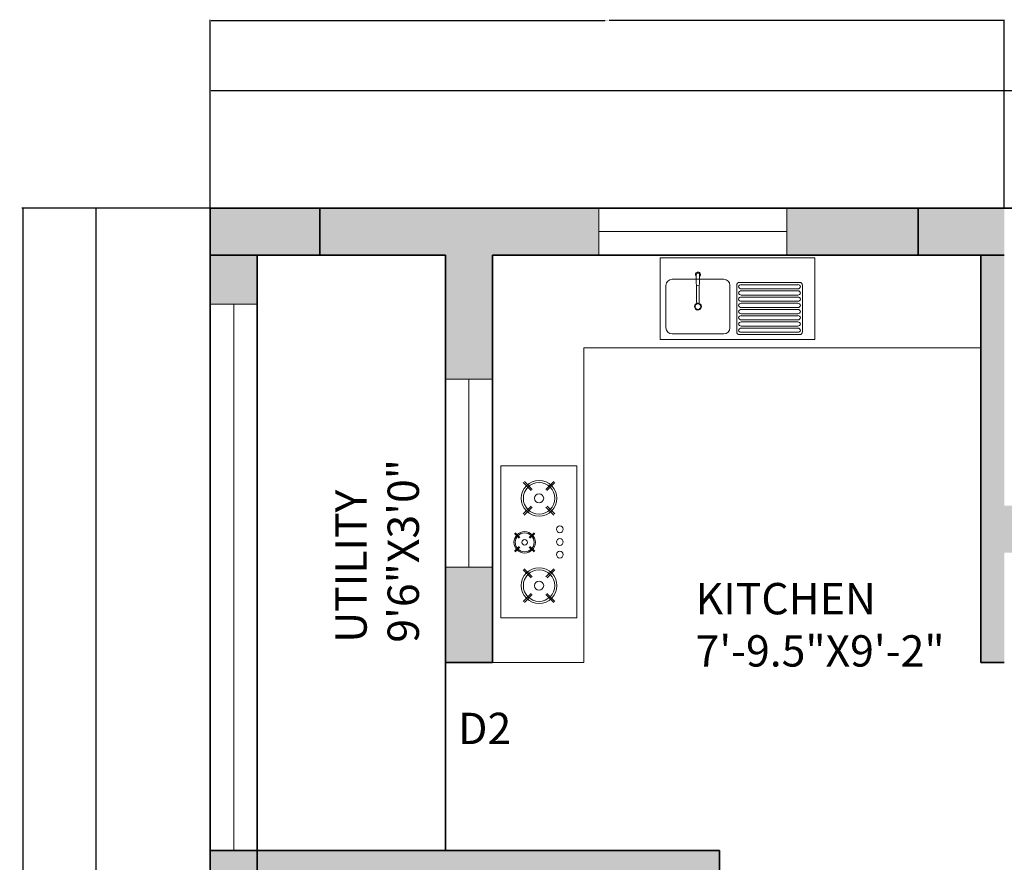
# Model space of a CAD drawing. Units: inches. Extents: x -9 to 505, y -680 to 48.
# Tile 16 of 17: x -9 to 179, y -114 to 48. Entities that reach past the tile are written whole.
import ezdxf

# ---------------------------------------------------------------- set-up
doc = ezdxf.new("R2010")
doc.units = ezdxf.units.IN
doc.header["$MEASUREMENT"] = 0
for name, color, linetype, lineweight in [('A-ANNO-DIMS', 2, 'Continuous', 18), ('A-ANNO-TEXT', 7, 'Continuous', 18), ('A-AREA-IDEN', 7, 'Continuous', 18), ('A-EQPM', 8, 'Continuous', 18), ('A-FLOR-CASE', 8, 'Continuous', 18), ('A-FLOR-FIXT', 9, 'Continuous', 18), ('A-FLOR-HRAL', 4, 'Continuous', 18), ('A-GLAZ', 4, 'Continuous', 18), ('A-WALL', 7, 'Continuous', 35), ('A-WALL-PATT', 251, 'Continuous', 13), ('S-CONC', 7, 'Continuous', 35), ('S-CONC-PATT', 18, 'Continuous', 13)]:
    doc.layers.add(name, color=color, linetype=linetype, lineweight=lineweight)
doc.styles.get("Standard").update_dxf_attribs({"font": 'arial.ttf'})
doc.dimstyles.get("Standard").update_dxf_attribs({"dimtxt": 0.18, "dimasz": 0.18, "dimexe": 0.18, "dimexo": 0.0625, "dimgap": 0.09, "dimtad": 0, "dimtih": 1, "dimtoh": 1, "dimdec": 0, "dimzin": 0, "dimdsep": 46, "dimlunit": 3, "dimtxsty": 'Standard', "dimcen": 0.09, "dimadec": 0, "dimazin": 0, "dimtfac": 1, "dimtdec": 0, "dimtofl": 0, "dimtmove": 0, "dimatfit": 3, "dimfxl": 1, "dimtolj": 1, "dimtzin": 0, "dimarcsym": 0})

# ---------------------------------------------------------------- blocks, each defined once
blk = doc.blocks.new('*D2')
at = {"layer": 'A-ANNO-DIMS', "color": 0, "lineweight": -2, "transparency": 16777216}
for p, q in [((27.26, 11.56), (27.26, 34.2)), ((27.44, 34.02), (235.29, 34.02)), ((468.58, 34.02), (260.74, 34.02)), ((468.76, 11.56), (468.76, 34.2))]:
    blk.add_line(p, q, dxfattribs=at)
at = {"layer": 'A-ANNO-DIMS', "color": 0, "transparency": 16777216}
for points in [[(27.44, 34.05), (27.44, 33.99), (27.26, 34.02)], [(468.58, 34.05), (468.58, 33.99), (468.76, 34.02)]]:
    blk.add_solid(points, dxfattribs=at)
at = {"layer": 'Defpoints', "color": 0, "transparency": 16777216}
for p in [(468.76, 34.02), (27.26, 11.5), (468.76, 11.5)]:
    blk.add_point(p, dxfattribs=at)
at = {"layer": 'A-ANNO-DIMS', "color": 0, "transparency": 16777216, "insert": (248.01, 34.02), "char_height": 6, "attachment_point": 5}
blk.add_mtext('\\A1;36\'-10"', dxfattribs=at)
blk = doc.blocks.new('*D3')
at = {"layer": 'A-ANNO-DIMS', "color": 0, "lineweight": -2, "transparency": 16777216}
for p, q in [((27.2, 11.5), (5.16, 11.5)), ((5.34, 11.32), (5.34, -330.86)), ((5.34, -679.32), (5.34, -337.14)), ((27.2, -679.5), (5.16, -679.5))]:
    blk.add_line(p, q, dxfattribs=at)
at = {"layer": 'A-ANNO-DIMS', "color": 0, "transparency": 16777216}
for points in [[(5.31, 11.32), (5.37, 11.32), (5.34, 11.5)], [(5.31, -679.32), (5.37, -679.32), (5.34, -679.5)]]:
    blk.add_solid(points, dxfattribs=at)
at = {"layer": 'Defpoints', "color": 0, "transparency": 16777216}
for p in [(27.26, 11.5), (5.34, -679.5), (27.26, -679.5)]:
    blk.add_point(p, dxfattribs=at)
at = {"layer": 'A-ANNO-DIMS', "color": 0, "transparency": 16777216, "insert": (5.34, -334), "char_height": 6, "attachment_point": 5}
blk.add_mtext('\\A1;57\'-7"', dxfattribs=at)
blk = doc.blocks.new('WIN-36')
for p, q in [((0, 36), (0, 0)), ((9, 36), (0, 36)), ((4.5, 36), (4.5, 2.23)), ((9, 0), (9, 36)), ((4.5, 2.23), (4.5, 0)), ((0, 0), (9, 0))]:
    blk.add_line(p, q)
blk = doc.blocks.new('SINK-SINGLE-DRAINBOARD')
for p, q in [((0, 0), (0, 15.65)), ((0, 15.65), (29.6, 15.65)), ((29.6, 0), (29.6, 15.65)), ((7.43, 11.55), (2.3, 11.55)), ((12.19, 11.55), (7.57, 11.55)), ((1.13, 10.39), (1.13, 2.25)), ((13.36, 2.25), (13.36, 10.39)), ((14.68, 10.42), (14.68, 1.51)), ((26.71, 10.96), (15.22, 10.96)), ((20.97, 10.52), (15.55, 10.52)), ((20.97, 9.72), (15.55, 9.72)), ((20.97, 10.52), (26.39, 10.52)), ((20.97, 9.72), (26.39, 9.72)), ((27.25, 10.42), (27.25, 1.51)), ((20.97, 9.34), (15.55, 9.34)), ((20.97, 8.53), (15.55, 8.53)), ((20.97, 8.15), (15.55, 8.15)), ((20.97, 9.34), (26.39, 9.34)), ((20.97, 8.53), (26.39, 8.53)), ((20.97, 8.15), (26.39, 8.15)), ((20.97, 7.34), (15.55, 7.34)), ((20.97, 6.96), (15.55, 6.96)), ((20.97, 6.15), (15.55, 6.15)), ((20.97, 5.77), (15.55, 5.77)), ((20.97, 7.34), (26.39, 7.34)), ((20.97, 6.96), (26.39, 6.96)), ((20.97, 6.15), (26.39, 6.15)), ((20.97, 5.77), (26.39, 5.77)), ((20.97, 4.96), (15.55, 4.96)), ((20.97, 4.58), (15.55, 4.58)), ((20.97, 3.78), (15.55, 3.78)), ((20.97, 4.96), (26.39, 4.96)), ((20.97, 4.58), (26.39, 4.58)), ((20.97, 3.78), (26.39, 3.78)), ((20.97, 3.4), (15.55, 3.4)), ((20.97, 2.59), (15.55, 2.59)), ((20.97, 2.21), (15.55, 2.21)), ((20.97, 3.4), (26.39, 3.4)), ((20.97, 2.59), (26.39, 2.59)), ((20.97, 2.21), (26.39, 2.21)), ((2.3, 1.09), (12.19, 1.09)), ((15.22, 0.97), (26.71, 0.97)), ((20.97, 1.4), (15.55, 1.4)), ((20.97, 1.4), (26.39, 1.4)), ((0, 0), (29.6, 0))]:
    blk.add_line(p, q)
for points in [[(6.92, 12.46), (6.92, 10.68)], [(7.57, 12.46), (7.57, 10.68)], [(7, 10.48), (7, 7.2)], [(7.49, 10.48), (7.49, 7.2)]]:
    blk.add_lwpolyline(points)
for radius in [0.674, 0.54]:
    blk.add_circle((7.25, 6.32), radius)
for centre, radius, start, end in [((2.3, 10.39), 1.17, 90, 180), ((7.25, 12.46), 0.485, 311.9018, 228.0982), ((7.25, 12.46), 0.324, 0, 180), ((12.19, 10.39), 1.17, 0, 90), ((7.25, 10.69), 0.324, 182.2198, 357.7802), ((15.22, 10.42), 0.54, 90, 180), ((15.55, 9.99), 0.54, 90, 165.5097), ((15.55, 10.26), 0.54, 194.4903, 270), ((26.39, 9.99), 0.54, 14.4903, 90), ((26.39, 10.26), 0.54, 270, 345.5097), ((26.71, 10.42), 0.54, 0, 90), ((15.55, 8.8), 0.54, 90, 165.5097), ((15.55, 9.07), 0.54, 194.4903, 270), ((15.55, 7.61), 0.54, 90, 165.5097), ((15.55, 7.88), 0.54, 194.4903, 270), ((26.39, 8.8), 0.54, 14.4903, 90), ((26.39, 9.07), 0.54, 270, 345.5097), ((26.39, 7.61), 0.54, 14.4903, 90), ((26.39, 7.88), 0.54, 270, 345.5097), ((7.25, 7.18), 0.244, 174.9463, 5.0537), ((15.55, 6.42), 0.54, 90, 165.5097), ((15.55, 6.69), 0.54, 194.4903, 270), ((15.55, 5.23), 0.54, 90, 165.5097), ((26.39, 6.42), 0.54, 14.4903, 90), ((26.39, 6.69), 0.54, 270, 345.5097), ((26.39, 5.23), 0.54, 14.4903, 90), ((15.55, 5.5), 0.54, 194.4903, 270), ((15.55, 4.05), 0.54, 90, 165.5097), ((15.55, 4.32), 0.54, 194.4903, 270), ((26.39, 5.5), 0.54, 270, 345.5097), ((26.39, 4.05), 0.54, 14.4903, 90), ((26.39, 4.32), 0.54, 270, 345.5097), ((2.3, 2.25), 1.17, 180, 270), ((12.19, 2.25), 1.17, 270, 0), ((15.55, 2.86), 0.54, 90, 165.5097), ((15.55, 3.13), 0.54, 194.4903, 270), ((15.55, 1.67), 0.54, 90, 165.5097), ((26.39, 2.86), 0.54, 14.4903, 90), ((26.39, 3.13), 0.54, 270, 345.5097), ((26.39, 1.67), 0.54, 14.4903, 90), ((15.22, 1.51), 0.54, 180, 270), ((15.55, 1.94), 0.54, 194.4903, 270), ((26.39, 1.94), 0.54, 270, 345.5097), ((26.71, 1.51), 0.54, 270, 0)]:
    blk.add_arc(centre, radius, start, end)
blk = doc.blocks.new('*D46')
at = {"layer": 'A-ANNO-DIMS', "color": 0, "lineweight": -2, "transparency": 16777216}
for p, q in [((27.2, 11.5), (-8.8, 11.5)), ((-8.62, 11.32), (-8.62, -137.57)), ((-8.62, -286.82), (-8.62, -137.93)), ((27.2, -287), (-8.8, -287))]:
    blk.add_line(p, q, dxfattribs=at)
at = {"layer": 'A-ANNO-DIMS', "color": 0, "transparency": 16777216}
for points in [[(-8.65, 11.32), (-8.59, 11.32), (-8.62, 11.5)], [(-8.65, -286.82), (-8.59, -286.82), (-8.62, -287)]]:
    blk.add_solid(points, dxfattribs=at)
at = {"layer": 'Defpoints', "color": 0, "transparency": 16777216}
for p in [(27.26, 11.5), (-8.62, -287), (27.26, -287)]:
    blk.add_point(p, dxfattribs=at)
at = {"layer": 'A-ANNO-DIMS', "color": 0, "transparency": 16777216, "insert": (-8.62, -137.75), "char_height": 0.18, "attachment_point": 5}
blk.add_mtext('\\A1;24\'-10 1/2"', dxfattribs=at)
blk = doc.blocks.new('*D47')
at = {"layer": 'A-ANNO-DIMS', "color": 0, "lineweight": -2, "transparency": 16777216}
for p, q in [((27.26, 11.56), (27.26, 47.56)), ((27.44, 47.38), (102.87, 47.38)), ((179.08, 47.38), (103.65, 47.38)), ((179.26, 11.56), (179.26, 47.56))]:
    blk.add_line(p, q, dxfattribs=at)
at = {"layer": 'A-ANNO-DIMS', "color": 0, "transparency": 16777216}
for points in [[(27.44, 47.41), (27.44, 47.35), (27.26, 47.38)], [(179.08, 47.41), (179.08, 47.35), (179.26, 47.38)]]:
    blk.add_solid(points, dxfattribs=at)
at = {"layer": 'Defpoints', "color": 0, "transparency": 16777216}
for p in [(179.26, 47.38), (27.26, 11.5), (179.26, 11.5)]:
    blk.add_point(p, dxfattribs=at)
at = {"layer": 'A-ANNO-DIMS', "color": 0, "transparency": 16777216, "insert": (103.26, 47.38), "char_height": 0.18, "attachment_point": 5}
blk.add_mtext('\\A1;12\'-8"', dxfattribs=at)

msp = doc.modelspace()

# ---------------------------------------------------------------- hatches: boundary and pattern name
at = {"layer": 'A-WALL-PATT'}
h = msp.add_hatch(color=256, dxfattribs=at)
h.dxf.hatch_style = 1
h.paths.add_polyline_path([(101.64, 11.5), (48.26, 11.5), (48.26, 2.5), (72.26, 2.5), (72.26, -21.25), (81.26, -21.25), (81.26, 2.5), (101.64, 2.5)])
h.paths.add_polyline_path([(36.26, 2.5), (27.26, 2.5), (27.26, -6.92), (36.26, -6.92)])
h.paths.add_polyline_path([(81.26, -57.25), (72.26, -57.25), (72.26, -75.5), (81.26, -75.5)])
h.paths.add_polyline_path([(162.76, 11.5), (137.64, 11.5), (137.64, 2.5), (162.76, 2.5)])
h.paths.add_polyline_path([(179.26, 2.5), (174.76, 2.5), (174.76, -75.5), (179.26, -75.5), (179.26, -54.5), (229.51, -54.5), (229.51, -45.5), (179.26, -45.5)])
h.paths.add_polyline_path([(382.26, -45.5), (332.26, -45.5), (332.26, 2.5), (327.76, 2.5), (327.76, -45.5), (277.51, -45.5), (277.51, -54.5), (327.76, -54.5), (327.76, -111.5), (332.26, -111.5), (332.26, -54.5), (382.26, -54.5)])
h.paths.add_polyline_path([(332.26, -128), (327.76, -128), (327.76, -207), (332.26, -207)])
h.paths.add_polyline_path([(124.76, -111.5), (36.26, -111.5), (36.26, -116), (120.26, -116), (120.26, -168.5), (179.26, -168.5), (179.26, -164), (124.76, -164)])
h.paths.add_polyline_path([(96.26, -164), (36.26, -164), (36.26, -152), (27.26, -152), (27.26, -208.88), (36.26, -208.88), (36.26, -168.5), (96.26, -168.5)])
h.paths.add_polyline_path([(36.26, -244.88), (27.26, -244.88), (27.26, -287), (36.26, -287)])
h.paths.add_polyline_path([(179.26, -204.5), (174.76, -204.5), (174.76, -287), (179.26, -287)])
h.paths.add_polyline_path([(257.26, -296), (248.26, -296), (248.26, -446), (269.26, -446), (269.26, -437), (257.26, -437)])
h.paths.add_polyline_path([(90.26, -296), (81.26, -296), (81.26, -348.67), (90.26, -348.67)])
h.paths.add_polyline_path([(90.26, -384.67), (81.26, -384.67), (81.26, -416), (90.26, -416)])
h.paths.add_polyline_path([(170.26, -452), (36.26, -452), (36.26, -456.5), (165.76, -456.5), (165.76, -504.5), (165.13, -504.5), (165.13, -509), (170.26, -509)])
h.paths.add_polyline_path([(141.76, -504.5), (36.26, -504.5), (36.26, -492.5), (27.26, -492.5), (27.26, -565.96), (36.26, -565.96), (36.26, -509), (141.76, -509)])
h.paths.add_polyline_path([(36.26, -601.96), (27.26, -601.96), (27.26, -658.5), (36.26, -658.5)])
h.paths.add_polyline_path([(170.26, -670.5), (170.26, -634.5), (222.76, -634.5), (222.76, -625.5), (165.76, -625.5), (165.76, -670.5), (36.26, -670.5), (36.26, -679.5), (170.26, -679.5)])
h.paths.add_polyline_path([(332.26, -616.5), (433.89, -616.5), (433.89, -612), (332.26, -612), (332.26, -610.56), (327.76, -610.56), (327.76, -625.5), (270.76, -625.5), (270.76, -634.5), (327.76, -634.5), (327.76, -658.5), (332.26, -658.5)])
h.paths.add_polyline_path([(459.76, -670.5), (336.76, -670.5), (336.76, -679.5), (459.76, -679.5)])
h.paths.add_polyline_path([(468.76, -545.74), (459.76, -545.74), (459.76, -612), (457.89, -612), (457.89, -616.5), (459.76, -616.5), (459.76, -658.5), (468.76, -658.5)])
h.paths.add_polyline_path([(332.26, -446), (327.76, -446), (327.76, -574.56), (332.26, -574.56)])
h.paths.add_polyline_path([(327.76, -437), (305.26, -437), (305.26, -446), (327.76, -446)])
h.paths.add_polyline_path([(459.76, -437), (348.76, -437), (348.76, -446), (459.76, -446)])
h.paths.add_polyline_path([(468.76, -458), (459.76, -458), (459.76, -509.74), (468.76, -509.74)])
h.paths.add_polyline_path([(468.76, -365), (459.76, -365), (459.76, -437), (468.76, -437)])
h.paths.add_polyline_path([(468.76, -299.6), (459.76, -299.6), (459.76, -344), (468.76, -344)])
h.paths.add_polyline_path([(468.76, -184.74), (459.76, -184.74), (459.76, -231), (401.26, -231), (401.26, -235.5), (459.76, -235.5), (459.76, -275.6), (468.76, -275.6)])
h.paths.add_polyline_path([(390.76, -356), (342.76, -356), (342.76, -365), (390.76, -365)])
h.paths.add_polyline_path([(459.76, -356), (405.76, -356), (405.76, -365), (459.76, -365)])
h.paths.add_polyline_path([(405.76, -296), (396.76, -296), (396.76, -356), (405.76, -356)])
h.paths.add_polyline_path([(336.76, -296), (327.76, -296), (327.76, -356), (336.76, -356)])
h.paths.add_polyline_path([(468.76, -9.5), (459.76, -9.5), (459.76, -45.5), (418.26, -45.5), (418.26, -54.5), (468.76, -54.5)])
h.paths.add_polyline_path([(468.76, -54.5), (459.76, -54.5), (459.76, -111.5), (468.76, -111.5)])
h.paths.add_polyline_path([(468.76, -128), (459.76, -128), (459.76, -148.74), (468.76, -148.74)])
at = {"layer": 'S-CONC-PATT'}
h = msp.add_hatch(color=256, dxfattribs=at)
h.dxf.hatch_style = 1
h.paths.add_polyline_path([(468.76, 11.5), (455.21, 11.5), (455.21, 2.5), (459.76, 2.5), (459.76, -9.5), (468.76, -9.5)])
h.paths.add_polyline_path([(179.26, 11.5), (162.76, 11.5), (162.76, 2.5), (179.26, 2.5)])
h.paths.add_polyline_path([(48.26, 11.5), (27.26, 11.5), (27.26, 2.5), (48.26, 2.5)])
h = msp.add_hatch(color=256, dxfattribs=at)
h.dxf.hatch_style = 1
h.paths.add_polyline_path([(36.26, -111.5), (27.26, -111.5), (27.26, -128), (36.26, -128)])

# ---------------------------------------------------------------- linework, layer by layer
at = {"layer": 'A-EQPM'}
for p, q in [((82.86, -37.88), (82.86, -66.97)), ((97.4, -37.88), (82.86, -37.88)), ((97.4, -66.97), (97.4, -37.88)), ((88.69, -42.56), (87.18, -41.05)), ((88.89, -42.36), (87.38, -40.85)), ((91.51, -42.36), (93.02, -40.85)), ((91.71, -42.56), (93.22, -41.05)), ((88.68, -45.57), (87.15, -47.07)), ((88.88, -45.77), (87.35, -47.27)), ((91.52, -45.77), (93.04, -47.27)), ((91.72, -45.57), (93.24, -47.07)), ((86.41, -51.71), (85.5, -50.8)), ((86.53, -51.59), (85.62, -50.68)), ((88.33, -51.58), (89.24, -50.67)), ((88.46, -51.7), (89.36, -50.79)), ((86.41, -53.28), (85.5, -54.19)), ((86.53, -53.4), (85.62, -54.31)), ((88.33, -53.41), (89.24, -54.32)), ((88.46, -53.29), (89.36, -54.2)), ((88.68, -59.28), (87.15, -57.78)), ((88.88, -59.08), (87.35, -57.58)), ((91.52, -59.08), (93.04, -57.58)), ((91.72, -59.28), (93.24, -57.78)), ((88.69, -62.29), (87.18, -63.8)), ((88.89, -62.49), (87.38, -64)), ((91.51, -62.49), (93.02, -64)), ((91.71, -62.29), (93.22, -63.8)), ((82.86, -66.97), (97.4, -66.97))]:
    msp.add_line(p, q, dxfattribs=at)
for centre, radius in [((90.2, -44.07), 3.42), ((90.2, -44.07), 3.01), ((90.2, -44.07), 0.881), ((87.44, -52.5), 2.05), ((87.44, -52.5), 1.81), ((94.17, -50), 0.646), ((87.44, -52.5), 0.529), ((94.17, -52.43), 0.646), ((94.17, -54.85), 0.646), ((90.2, -60.78), 3.42), ((90.2, -60.78), 3.01), ((90.2, -60.78), 0.881)]:
    msp.add_circle(centre, radius, dxfattribs=at)
at = {"layer": 'A-FLOR-CASE'}
for p, q in [((98.76, -75.5), (98.76, -15.24)), ((98.76, -15.24), (174.76, -15.24)), ((81.26, -75.5), (98.76, -75.5))]:
    msp.add_line(p, q, dxfattribs=at)
at = {"layer": 'A-FLOR-HRAL'}
for p, q in [((36.26, -6.92), (27.26, -6.92)), ((27.26, -6.92), (27.26, -111.5)), ((31.76, -6.92), (31.76, -111.5)), ((36.26, -111.5), (36.26, -6.92)), ((27.26, -111.5), (36.26, -111.5))]:
    msp.add_line(p, q, dxfattribs=at)
at = {"layer": 'A-GLAZ'}
for p, q in [((101.64, 11.5), (137.64, 11.5)), ((101.64, 2.5), (101.64, 11.5)), ((137.64, 11.5), (137.64, 2.5)), ((101.64, 7), (137.64, 7)), ((137.64, 2.5), (101.64, 2.5))]:
    msp.add_line(p, q, dxfattribs=at)
at = {"layer": 'A-WALL'}
for p, q in [((27.26, 11.5), (27.26, -679.5)), ((27.26, 11.5), (468.76, 11.5)), ((27.26, 2.5), (72.26, 2.5)), ((36.26, 2.5), (36.26, -164)), ((72.26, 2.5), (72.26, -111.5)), ((81.26, 2.5), (81.26, -75.5)), ((81.26, 2.5), (179.26, 2.5)), ((174.76, 2.5), (174.76, -75.5)), ((81.26, -75.5), (72.26, -75.5)), ((174.76, -75.5), (179.26, -75.5)), ((27.26, -111.5), (124.76, -111.5)), ((124.76, -111.5), (124.76, -164))]:
    msp.add_line(p, q, dxfattribs=at)
at = {"layer": 'S-CONC'}
for p, q in [((48.26, 2.5), (48.26, 11.5)), ((162.76, 2.5), (162.76, 11.5))]:
    msp.add_line(p, q, dxfattribs=at)

# ---------------------------------------------------------------- block references
at = {"layer": 'A-FLOR-FIXT'}
msp.add_blockref('SINK-SINGLE-DRAINBOARD', (113.36, -13.69), dxfattribs=at)
at = {"layer": 'A-GLAZ'}
msp.add_blockref('WIN-36', (72.26, -57.25), dxfattribs=at)

# ---------------------------------------------------------------- texts
at = {"layer": 'A-ANNO-TEXT', "insert": (74.7, -85.12), "char_height": 6, "attachment_point": 1}
msp.add_mtext('D2', dxfattribs=at)
at = {"layer": 'A-AREA-IDEN', "insert": (51.2, -71.71), "char_height": 6, "attachment_point": 1, "rotation": 90}
msp.add_mtext('UTILITY\\P9\'6"X3\'0"', dxfattribs=at)
at = {"layer": 'A-AREA-IDEN', "insert": (120.16, -60.28), "char_height": 6, "attachment_point": 1}
msp.add_mtext('KITCHEN\\P7\'-9.5"X9\'-2"', dxfattribs=at)

# ---------------------------------------------------------------- dimensions: what is measured, and where the dimension line sits
at = {"layer": 'A-ANNO-DIMS'}
for base, p1, p2, override, picture, middle in [((179.26, 47.38), (27.26, 11.5), (179.26, 11.5), {"dimdec": 1, "dimlfac": 1, "dimrnd": 0, "dimzin": 1, "dimdsep": 46, "dimlunit": 4, "dimfrac": 2}, '*D47', (103.26, 47.38)), ((468.76354104, 34.01880442), (27.26354104, 11.49914079), (468.76354104, 11.49914079), {"dimtxt": 6, "dimclrd": 0, "dimclre": 0, "dimclrt": 0}, '*D2', (248.01354104, 34.01880442))]:
    dim = msp.add_linear_dim(base=base, p1=p1, p2=p2, dimstyle='Standard', override=override, dxfattribs=at)
    dim.commit()
    dim.dimension.update_dxf_attribs({"geometry": picture, "text_midpoint": middle})
for base, p2, override, picture, middle in [((-8.62, -287), (27.26, -287), {"dimdec": 1, "dimlfac": 1, "dimrnd": 0, "dimzin": 1, "dimdsep": 46, "dimlunit": 4, "dimfrac": 2}, '*D46', (-8.62, -137.75)), ((5.34, -679.5), (27.26, -679.5), {"dimtxt": 6, "dimclrd": 0, "dimclre": 0, "dimclrt": 0}, '*D3', (5.34, -334))]:
    dim = msp.add_linear_dim(base=base, p1=(27.26, 11.5), p2=p2, angle=90, dimstyle='Standard', override=override, dxfattribs=at)
    dim.commit()
    dim.dimension.update_dxf_attribs({"geometry": picture, "text_midpoint": middle})

doc.saveas('drawing.dxf')
